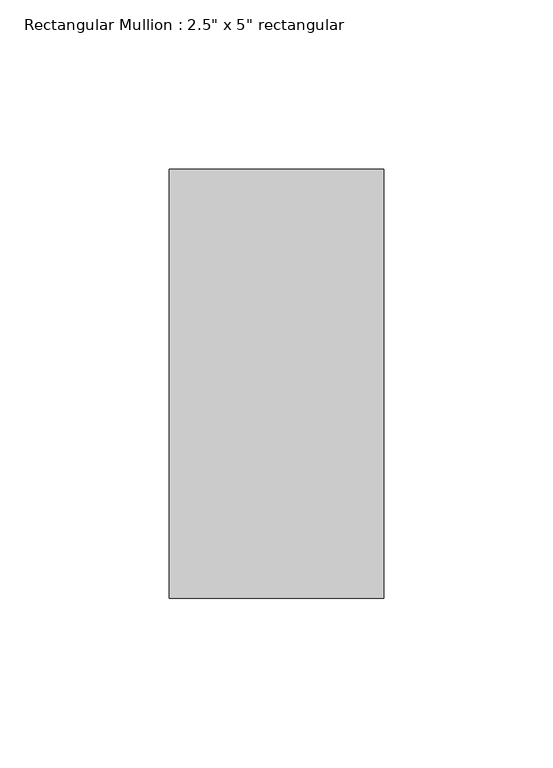
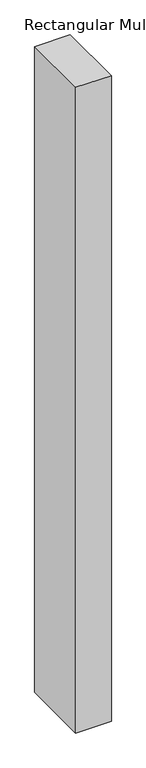
"""IFC4 building model written with IfcOpenShell, lengths in millimetres: member geometry."""

from ifc_helpers import new_model, si_unit, frame, origin, place, context, project, spatial, polyline, outline, extrude, source, transform, mapped, element, save


def member_2b49869a(model_context):
    return source(origin(), model_context, "Body", "SweptSolid", [
        extrude(outline(polyline([(31.75, 63.5), (31.75, -63.5), (-31.75, -63.5), (-31.75, 63.5), (31.75, 63.5)])), frame((0.0, 0.0, -1219.2), z_axis=(0.0, 0.0, 1.0), x_axis=(1.0, 0.0, 0.0)), (0.0, 0.0, 1.0), 1219.2),
    ])


if __name__ == "__main__":
    model = new_model("IFC4")
    model_context = context("Model", 3, world=origin())
    ifc_project = project(units=[si_unit("LENGTHUNIT", "METRE", prefix="MILLI")], contexts=[model_context])
    site = spatial("IfcSite", under=ifc_project)
    building = spatial("IfcBuilding", under=site)
    placement = place(None, origin())
    member_shape = member_2b49869a(model_context)
    element("IfcMember", 1, ObjectType="Rectangular Mullion : 2.5\" x 5\" rectangular", at=placement, inside=building, context=model_context, shape_type="MappedRepresentation", body=[
        mapped(member_shape, transform((0.0, 0.0, 0.0), x_axis=(1.0, 0.0, 0.0), y_axis=(0.0, 1.0, 0.0), z_axis=(0.0, 0.0, 1.0))),
    ])
    save(model, "model.ifc")

# Revit data of these elements
# Type "Rectangular Mullion : 2.5\" x 5\" rectangular"
#   built-in parameter 1007304 = 0.416667 (stored number, unit not read)
#   built-in parameter 1007301 = 0.104167 (stored number, unit not read)
#   built-in parameter 1007300 = 0.104167 (stored number, unit not read)
# Element 1 (IfcMember, "Rectangular Mullion : 2.5\" x 5\" rectangular")
#   Materials on its faces: "Aluminum"
# Materials
#   "Aluminum": class "Metal", colour RGB 247 247 247, transparency 0, Description = "Aluminum 6061", Cost = 0
